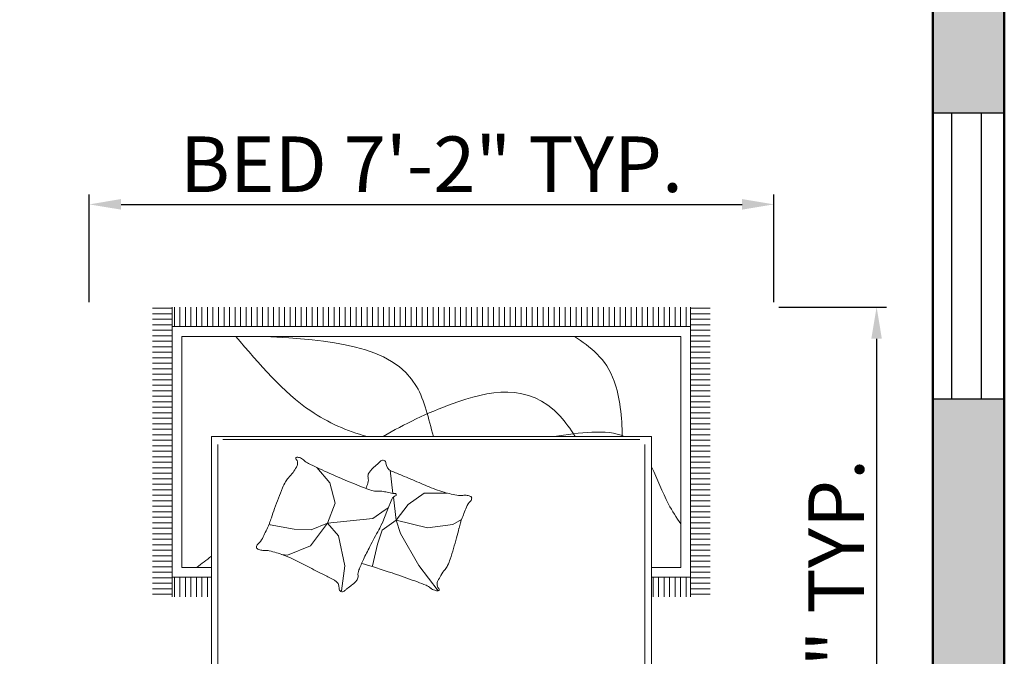
# Model space of a CAD drawing. Units: inches. Extents: x -7 to 1228, y -146 to 1091.
# Tile 84 of 88: x 1003 to 1127, y 611 to 691. Entities that reach past the tile are written whole.
import ezdxf

# ---------------------------------------------------------------- set-up
doc = ezdxf.new("R2010")
doc.units = ezdxf.units.IN
for name, color, linetype, lineweight in [('A-ANNO-DIMS', 2, 'Continuous', 18), ('A-FURN', 8, 'Continuous', 18), ('A-GLAZ', 175, 'Continuous', 25), ('A-WALL', 7, 'Continuous', 50), ('A-WALL-PATT', 251, 'Continuous', 13)]:
    doc.layers.add(name, color=color, linetype=linetype, lineweight=lineweight)
doc.styles.add('DIM_FONT', font='SIMPLEX.shx', dxfattribs={"width": 0.8})
doc.styles.get("Standard").update_dxf_attribs({"font": 'arial.ttf'})
doc.dimstyles.new('ISO-25', dxfattribs={"dimtxt": 7, "dimasz": 4, "dimexe": 1.25, "dimexo": 0.625, "dimtad": 1, "dimdec": 1, "dimlunit": 3, "dimtxsty": 'Standard', "dimcen": 2.5, "dimadec": 0, "dimazin": 0, "dimtfac": 1, "dimtdec": 1, "dimtmove": 1, "dimatfit": 3, "dimfxl": 1, "dimarcsym": 0})

# ---------------------------------------------------------------- blocks, each defined once
blk = doc.blocks.new('A$C4F634EDD')
for p, q in [((0.5, 0.5295), (0.5, 2.6295)), ((2.3, 2.6295), (2.3, 0.5295)), ((0.5258, 2.121), (0.5258, 0.5617)), ((2.2716, 0.5617), (2.2716, 1.7136)), ((0.2586, 1.1753), (0.3386, 1.1753)), ((0.3386, 0), (0.3386, 1.1852)), ((0.3486, 1.1052), (0.3486, 1.1852)), ((0.3711, 1.1052), (0.3711, 1.1852)), ((0.3936, 1.1052), (0.3936, 1.1852)), ((0.4161, 1.1052), (0.4161, 1.1852)), ((0.4386, 1.1052), (0.4386, 1.1852)), ((0.4611, 1.1052), (0.4611, 1.1852)), ((0.4836, 1.1052), (0.4836, 1.1852)), ((2.3061, 1.1052), (2.3061, 1.1852)), ((2.3286, 1.1052), (2.3286, 1.1852)), ((2.3511, 1.1052), (2.3511, 1.1852)), ((2.3736, 1.1052), (2.3736, 1.1852)), ((2.3961, 1.1052), (2.3961, 1.1852)), ((2.4186, 1.1052), (2.4186, 1.1852)), ((2.4411, 1.1052), (2.4411, 1.1852)), ((2.4588, 1.1852), (2.4588, 0)), ((2.4588, 1.1753), (2.5388, 1.1753)), ((0.2586, 1.1528), (0.3386, 1.1528)), ((0.2586, 1.1303), (0.3386, 1.1303)), ((1.031, 1.1612), (1.0448, 1.0581)), ((1.4276, 1.1611), (1.3484, 1.0571)), ((2.4588, 1.1528), (2.5388, 1.1528)), ((2.4588, 1.1303), (2.5388, 1.1303)), ((0.2586, 1.1078), (0.3386, 1.1078)), ((0.3386, 1.1052), (0.5, 1.1052)), ((2.3, 1.1052), (2.4588, 1.1052)), ((2.4588, 1.1078), (2.5388, 1.1078)), ((0.2586, 1.0853), (0.3386, 1.0853)), ((0.2586, 1.0628), (0.3386, 1.0628)), ((0.3786, 1.0652), (0.5, 1.0652)), ((0.3786, 0.12), (0.3786, 1.0652)), ((1.0448, 1.0581), (1.019, 0.936)), ((1.1784, 0.9702), (1.1586, 1.0591)), ((1.3484, 1.0571), (1.2733, 0.9268)), ((2.3, 1.0652), (2.4188, 1.0652)), ((2.4188, 1.0652), (2.4188, 0.12)), ((2.4588, 1.0853), (2.5388, 1.0853)), ((2.4588, 1.0628), (2.5388, 1.0628)), ((0.2586, 1.0403), (0.3386, 1.0403)), ((0.2586, 1.0178), (0.3386, 1.0178)), ((0.8108, 1.0151), (0.7868, 1.0117)), ((0.9054, 0.9773), (0.8108, 1.0151)), ((2.4588, 1.0403), (2.5388, 1.0403)), ((2.4588, 1.0178), (2.5388, 1.0178)), ((0.2586, 0.9953), (0.3386, 0.9953)), ((0.2586, 0.9728), (0.3386, 0.9728)), ((0.9743, 0.8845), (0.9054, 0.9773)), ((1.1982, 0.9129), (1.1784, 0.9702)), ((2.4588, 0.9953), (2.5388, 0.9953)), ((2.4588, 0.9728), (2.5388, 0.9728)), ((0.2586, 0.9503), (0.3386, 0.9503)), ((0.2586, 0.9278), (0.3386, 0.9278)), ((1.019, 0.936), (0.9743, 0.8845)), ((1.2733, 0.9268), (1.2555, 0.8715)), ((2.4588, 0.9503), (2.5388, 0.9503)), ((2.4588, 0.9278), (2.5388, 0.9278)), ((0.2586, 0.9053), (0.3386, 0.9053)), ((0.7403, 0.8913), (0.737, 0.8849)), ((0.8384, 0.9085), (0.7403, 0.8913)), ((0.9072, 0.912), (0.8384, 0.9085)), ((0.9743, 0.8845), (0.9072, 0.912)), ((1.2555, 0.8715), (1.1982, 0.9129)), ((1.2555, 0.8715), (1.384, 0.9031)), ((1.384, 0.9031), (1.4868, 0.8892)), ((1.4868, 0.8892), (1.5228, 0.8692)), ((2.4588, 0.9053), (2.5388, 0.9053)), ((0.2586, 0.8828), (0.3386, 0.8828)), ((0.2586, 0.8603), (0.3386, 0.8603)), ((0.9743, 0.8845), (1.0052, 0.802)), ((0.9743, 0.8845), (1.16, 0.8656)), ((1.16, 0.8656), (1.2099, 0.8295)), ((1.1973, 0.8853), (1.2203, 0.829)), ((1.2555, 0.8715), (1.2437, 0.7773)), ((1.2555, 0.8715), (1.3049, 0.8082)), ((2.4588, 0.8828), (2.5388, 0.8828)), ((2.4588, 0.8603), (2.5388, 0.8603)), ((0.2586, 0.8378), (0.3386, 0.8378)), ((0.2586, 0.8153), (0.3386, 0.8153)), ((1.2099, 0.8295), (1.222, 0.8209)), ((1.2203, 0.829), (1.2381, 0.7855)), ((1.3049, 0.8082), (1.3701, 0.7608)), ((2.4588, 0.8378), (2.5388, 0.8378)), ((2.4588, 0.8153), (2.5388, 0.8153)), ((0.2586, 0.7928), (0.3386, 0.7928)), ((0.2586, 0.7703), (0.3386, 0.7703)), ((1.0052, 0.802), (0.9846, 0.7194)), ((2.4588, 0.7928), (2.5388, 0.7928)), ((2.4588, 0.7703), (2.5388, 0.7703)), ((0.2586, 0.7478), (0.3386, 0.7478)), ((0.2586, 0.7253), (0.3386, 0.7253)), ((1.2419, 0.7626), (1.23, 0.668)), ((1.3701, 0.7608), (1.463, 0.7608)), ((2.4588, 0.7478), (2.5388, 0.7478)), ((2.4588, 0.7253), (2.5388, 0.7253)), ((0.2586, 0.7028), (0.3386, 0.7028)), ((0.9846, 0.7194), (0.931, 0.6569)), ((2.4588, 0.7028), (2.5388, 0.7028)), ((0.2586, 0.6803), (0.3386, 0.6803)), ((0.2586, 0.6578), (0.3386, 0.6578)), ((2.4588, 0.6803), (2.5388, 0.6803)), ((2.4588, 0.6578), (2.5388, 0.6578)), ((0.2586, 0.6353), (0.3386, 0.6353)), ((0.2586, 0.6128), (0.3386, 0.6128)), ((2.4588, 0.6353), (2.5388, 0.6353)), ((2.4588, 0.6128), (2.5388, 0.6128)), ((0.2586, 0.5903), (0.3386, 0.5903)), ((0.2586, 0.5678), (0.3386, 0.5678)), ((2.4588, 0.5903), (2.5388, 0.5903)), ((2.4588, 0.5678), (2.5388, 0.5678)), ((0.2586, 0.5453), (0.3386, 0.5453)), ((2.3, 0.5295), (0.5, 0.5295)), ((0.5458, 0.5417), (2.2516, 0.5417)), ((2.4588, 0.5453), (2.5388, 0.5453)), ((0.2586, 0.5228), (0.3386, 0.5228)), ((0.2586, 0.5003), (0.3386, 0.5003)), ((2.4588, 0.5228), (2.5388, 0.5228)), ((2.4588, 0.5003), (2.5388, 0.5003)), ((0.2586, 0.4778), (0.3386, 0.4778)), ((0.2586, 0.4553), (0.3386, 0.4553)), ((2.4588, 0.4778), (2.5388, 0.4778)), ((2.4588, 0.4553), (2.5388, 0.4553)), ((0.2586, 0.4328), (0.3386, 0.4328)), ((0.2586, 0.4103), (0.3386, 0.4103)), ((2.4588, 0.4328), (2.5388, 0.4328)), ((2.4588, 0.4103), (2.5388, 0.4103)), ((0.2586, 0.3878), (0.3386, 0.3878)), ((0.2586, 0.3653), (0.3386, 0.3653)), ((2.4588, 0.3878), (2.5388, 0.3878)), ((2.4588, 0.3653), (2.5388, 0.3653)), ((0.2586, 0.3428), (0.3386, 0.3428)), ((2.4588, 0.3428), (2.5388, 0.3428)), ((0.2586, 0.3203), (0.3386, 0.3203)), ((0.2586, 0.2978), (0.3386, 0.2978)), ((2.4588, 0.3203), (2.5388, 0.3203)), ((2.4588, 0.2978), (2.5388, 0.2978)), ((0.2586, 0.2753), (0.3386, 0.2753)), ((0.2586, 0.2528), (0.3386, 0.2528)), ((2.4588, 0.2753), (2.5388, 0.2753)), ((2.4588, 0.2528), (2.5388, 0.2528)), ((0.2586, 0.2303), (0.3386, 0.2303)), ((0.2586, 0.2078), (0.3386, 0.2078)), ((2.4588, 0.2303), (2.5388, 0.2303)), ((2.4588, 0.2078), (2.5388, 0.2078)), ((0.2586, 0.1853), (0.3386, 0.1853)), ((0.2586, 0.1628), (0.3386, 0.1628)), ((2.4588, 0.1853), (2.5388, 0.1853)), ((2.4588, 0.1628), (2.5388, 0.1628)), ((0.2586, 0.1403), (0.3386, 0.1403)), ((2.4588, 0.1403), (2.5388, 0.1403)), ((0.2586, 0.1178), (0.3386, 0.1178)), ((0.2586, 0.0953), (0.3386, 0.0953)), ((2.4188, 0.12), (0.3786, 0.12)), ((2.4588, 0.1178), (2.5388, 0.1178)), ((2.4588, 0.0953), (2.5388, 0.0953)), ((0.2586, 0.0728), (0.3386, 0.0728)), ((0.2586, 0.0503), (0.3386, 0.0503)), ((2.4588, 0.08), (0.3386, 0.08)), ((0.3486, 0), (0.3486, 0.08)), ((0.3711, 0), (0.3711, 0.08)), ((0.3936, 0), (0.3936, 0.08)), ((0.4161, 0), (0.4161, 0.08)), ((0.4386, 0), (0.4386, 0.08)), ((0.4611, 0), (0.4611, 0.08)), ((0.4836, 0), (0.4836, 0.08)), ((0.5061, 0), (0.5061, 0.08)), ((0.5286, 0), (0.5286, 0.08)), ((0.5511, 0), (0.5511, 0.08)), ((0.5736, 0), (0.5736, 0.08)), ((0.5961, 0), (0.5961, 0.08)), ((0.6186, 0), (0.6186, 0.08)), ((0.6411, 0), (0.6411, 0.08)), ((0.6636, 0), (0.6636, 0.08)), ((0.6861, 0), (0.6861, 0.08)), ((0.7086, 0), (0.7086, 0.08)), ((0.7311, 0), (0.7311, 0.08)), ((0.7536, 0), (0.7536, 0.08)), ((0.7761, 0), (0.7761, 0.08)), ((0.7986, 0), (0.7986, 0.08)), ((0.8211, 0), (0.8211, 0.08)), ((0.8436, 0), (0.8436, 0.08)), ((0.8661, 0), (0.8661, 0.08)), ((0.8886, 0), (0.8886, 0.08)), ((0.9111, 0), (0.9111, 0.08)), ((0.9336, 0), (0.9336, 0.08)), ((0.9561, 0), (0.9561, 0.08)), ((0.9786, 0), (0.9786, 0.08)), ((1.0011, 0), (1.0011, 0.08)), ((1.0236, 0), (1.0236, 0.08)), ((1.0461, 0), (1.0461, 0.08)), ((1.0686, 0), (1.0686, 0.08)), ((1.0911, 0), (1.0911, 0.08)), ((1.1136, 0), (1.1136, 0.08)), ((1.1361, 0), (1.1361, 0.08)), ((1.1586, 0), (1.1586, 0.08)), ((1.1811, 0), (1.1811, 0.08)), ((1.2036, 0), (1.2036, 0.08)), ((1.2261, 0), (1.2261, 0.08)), ((1.2486, 0), (1.2486, 0.08)), ((1.2711, 0), (1.2711, 0.08)), ((1.2936, 0), (1.2936, 0.08)), ((1.3161, 0), (1.3161, 0.08)), ((1.3386, 0), (1.3386, 0.08)), ((1.3611, 0), (1.3611, 0.08)), ((1.3836, 0), (1.3836, 0.08)), ((1.4061, 0), (1.4061, 0.08)), ((1.4286, 0), (1.4286, 0.08)), ((1.4511, 0), (1.4511, 0.08)), ((1.4736, 0), (1.4736, 0.08)), ((1.4961, 0), (1.4961, 0.08)), ((1.5186, 0), (1.5186, 0.08)), ((1.5411, 0), (1.5411, 0.08)), ((1.5636, 0), (1.5636, 0.08)), ((1.5861, 0), (1.5861, 0.08)), ((1.6086, 0), (1.6086, 0.08)), ((1.6311, 0), (1.6311, 0.08)), ((1.6536, 0), (1.6536, 0.08)), ((1.6761, 0), (1.6761, 0.08)), ((1.6986, 0), (1.6986, 0.08)), ((1.7211, 0), (1.7211, 0.08)), ((1.7436, 0), (1.7436, 0.08)), ((1.7661, 0), (1.7661, 0.08)), ((1.7886, 0), (1.7886, 0.08)), ((1.8111, 0), (1.8111, 0.08)), ((1.8336, 0), (1.8336, 0.08)), ((1.8561, 0), (1.8561, 0.08)), ((1.8786, 0), (1.8786, 0.08)), ((1.9011, 0), (1.9011, 0.08)), ((1.9236, 0), (1.9236, 0.08)), ((1.9461, 0), (1.9461, 0.08)), ((1.9686, 0), (1.9686, 0.08)), ((1.9911, 0), (1.9911, 0.08)), ((2.0136, 0), (2.0136, 0.08)), ((2.0361, 0), (2.0361, 0.08)), ((2.0586, 0), (2.0586, 0.08)), ((2.0811, 0), (2.0811, 0.08)), ((2.1036, 0), (2.1036, 0.08)), ((2.1261, 0), (2.1261, 0.08)), ((2.1486, 0), (2.1486, 0.08)), ((2.1711, 0), (2.1711, 0.08)), ((2.1936, 0), (2.1936, 0.08)), ((2.2161, 0), (2.2161, 0.08)), ((2.2386, 0), (2.2386, 0.08)), ((2.2611, 0), (2.2611, 0.08)), ((2.2836, 0), (2.2836, 0.08)), ((2.3061, 0), (2.3061, 0.08)), ((2.3286, 0), (2.3286, 0.08)), ((2.3511, 0), (2.3511, 0.08)), ((2.3736, 0), (2.3736, 0.08)), ((2.3961, 0), (2.3961, 0.08)), ((2.4186, 0), (2.4186, 0.08)), ((2.4411, 0), (2.4411, 0.08)), ((2.4588, 0.0728), (2.5388, 0.0728)), ((2.4588, 0.0503), (2.5388, 0.0503)), ((0.2586, 0.0278), (0.3386, 0.0278)), ((0.2586, 0.0053), (0.3386, 0.0053)), ((2.4588, 0.0278), (2.5388, 0.0278)), ((2.4588, 0.0053), (2.5388, 0.0053))]:
    blk.add_line(p, q)
for centre, radius, start, end in [((0.9863, 1.1494), 0.0359, 297.2902, 3.2455), ((1.0348, 1.1521), 0.0127, 51.1864, 183.2455), ((0.9991, 1.1077), 0.0697, 45.8726, 51.1864), ((1.0791, 1.1902), 0.0452, 225.8726, 232.4713), ((1.2846, 1.4577), 0.3825, 232.4713, 233.7837), ((0.6683, 0.6162), 0.6605, 52.7849, 53.7837), ((0.9362, 0.9689), 0.2176, 46.4776, 52.7849), ((1.0543, 1.9106), 0.8371, 290.1287, 292.7069), ((1.3469, 1.2115), 0.0792, 292.7069, 308.5854), ((1.4338, 1.1026), 0.0601, 110.3452, 128.5854), ((1.4251, 1.1259), 0.0352, 86.0516, 110.3452), ((1.4996, 1.1284), 0.0771, 169.5926, 177.2714), ((1.4378, 1.1314), 0.0153, 177.2714, 194.5709), ((1.4611, 1.1374), 0.0393, 194.5709, 206.8179), ((1.4376, 1.1398), 0.0142, 126.5792, 169.5926), ((1.4273, 1.1567), 0.00443, 13.2808, 86.0516), ((1.4254, 1.1562), 0.0063, 306.5792, 13.2808), ((1.8575, -0.7096), 2.0162, 116.4147, 117.4999), ((-0.4173, 3.8699), 3.0972, 296.4147, 297.2902), ((1.0327, 1.0706), 0.0774, 35.8936, 46.4776), ((1.0771, 1.1027), 0.0226, 351.9508, 35.8936), ((1.1449, 1.0931), 0.0458, 171.9508, 202.4162), ((0.2266, 4.0657), 3.145, 286.6085, 289.0836), ((-0.4107, 5.9078), 5.0942, 289.0836, 290.1287), ((1.7401, 1.2785), 0.352, 206.8179, 210.9056), ((1.6045, 1.1973), 0.194, 210.9056, 219.7005), ((-1.8336, 6.2238), 5.8383, 297.49208, 297.84822), ((3.744, -4.3336), 6.1019, 117.49986, 117.84822), ((2.032, 1.4591), 1.0054, 202.4162, 205.0529), ((1.0922, 1.1636), 0.1166, 280.7366, 286.6085), ((1.3929, 1.0217), 0.081, 26.0735, 39.7005), ((1.2892, 0.9709), 0.1965, 17.8396, 26.0735), ((0.6422, 1.4168), 0.43, 282.6252, 290.7486), ((0.5736, 1.5979), 0.6236, 290.7486, 297.4921), ((2.6493, 1.7476), 1.6868, 205.0529, 207.0884), ((-0.4304, 0.4175), 2.003, 15.2625, 17.8396), ((0.6894, 0.9832), 0.0058, 121.6917, 179.0386), ((0.7004, 0.983), 0.0168, 179.0386, 229.4914), ((0.7131, 0.9448), 0.0509, 103.0402, 121.6917), ((0.6405, 0.9128), 0.0755, 26.3332, 49.4914), ((0.7152, 0.9361), 0.0599, 86.6119, 103.0402), ((0.7224, 1.0587), 0.063, 266.6119, 282.6252), ((2.541, 1.6922), 1.5652, 207.0884, 209.936), ((-1.6775, -0.2344), 2.6619, 25.1732, 26.3332), ((-0.0881, 0.5109), 1.6481, 13.841, 15.2625), ((0.5689, 0.8213), 0.1798, 20.7081, 25.1732), ((0.9989, 0.8042), 0.2143, 22.2355, 29.936), ((2.0418, 1.0357), 0.5454, 193.841, 196.3122), ((0.2268, 0.692), 0.5454, 18.2369, 20.7081), ((2.3102, 1.3785), 1.6481, 198.2369, 199.6584), ((1.6908, 0.933), 0.1798, 196.3122, 200.7773), ((4.0115, 1.8135), 2.6619, 200.7773, 201.9373), ((2.6444, 1.4979), 2.003, 199.6584, 202.2355), ((1.6124, 0.8472), 0.0755, 201.9373, 225.0955), ((1.2594, 0.7942), 0.0231, 202.2355, 252.8133), ((1.2512, 0.7678), 0.00467, 289.3799, 72.8133), ((1.5721, 0.3449), 0.43, 98.2293, 106.3527), ((1.5195, 0.708), 0.063, 82.216, 98.2293), ((1.5362, 0.8298), 0.0599, 262.216, 278.6443), ((1.5375, 0.8209), 0.0509, 278.6443, 297.2959), ((1.5473, 0.7819), 0.0168, 354.6428, 45.0955), ((1.5582, 0.7808), 0.0058, 297.2959, 354.6428), ((0.9722, 0.8143), 0.1965, 202.2355, 210.4694), ((2.2689, -2.1899), 3.145, 111.0043, 113.4795), ((0.1831, 0.4093), 1.0054, 18.0203, 19.3448), ((1.1834, 0.6373), 0.1166, 98.1216, 111.0043), ((1.1763, 0.687), 0.0663, 85.4882, 98.1216), ((1.1871, 0.8241), 0.0712, 265.4882, 277.6784), ((1.1727, 0.9313), 0.1794, 277.6784, 284.8807), ((1.2689, 0.569), 0.1955, 97.9822, 104.8807), ((1.2465, 0.729), 0.034, 85.7407, 97.9822), ((1.2497, 0.772), 0.0092, 265.7407, 289.3799), ((3.6722, -4.6377), 5.8383, 113.0962, 113.45234), ((1.6266, 0.159), 0.6236, 106.3527, 113.0962), ((0.8727, 0.7557), 0.081, 210.4694, 224.0964), ((0.6752, 0.5644), 0.194, 35.3015, 44.0964), ((3.0455, -3.9778), 5.0942, 113.4795, 114.5246), ((1.0957, 0.7061), 0.0458, 347.5549, 18.0203), ((1.1625, 0.6914), 0.0226, 167.5549, 211.4977), ((2.4404, -2.1823), 3.0972, 112.0188, 112.8944), ((0.5234, 2.5582), 2.0162, 292.0188, 293.104), ((-1.0798, 6.3161), 6.1019, 293.10398, 293.45234), ((0.5462, 0.4731), 0.352, 31.2138, 35.3015), ((0.8136, 0.6351), 0.0393, 18.9668, 31.2138), ((0.8364, 0.6429), 0.0153, 1.6673, 18.9668), ((1.2784, -0.1047), 0.8371, 114.5246, 117.1028), ((1.2092, 0.72), 0.0774, 211.4977, 222.0817), ((1.3133, 0.814), 0.2176, 222.0817, 228.389), ((1.6074, 1.1451), 0.6605, 228.389, 229.3878), ((1.2495, 0.6379), 0.0359, 112.8944, 178.8496), ((0.8506, 0.6191), 0.0063, 130.9751, 197.6767), ((0.8488, 0.6185), 0.00443, 197.6767, 270.4475), ((0.8372, 0.6345), 0.0142, 310.9751, 353.9885), ((0.8486, 0.6493), 0.0352, 270.4475, 294.7411), ((0.7746, 0.6411), 0.0771, 353.9885, 1.6673), ((0.8382, 0.6719), 0.0601, 294.7411, 312.9813), ((0.9332, 0.57), 0.0792, 117.1028, 132.9813), ((0.9284, 0.3533), 0.3825, 48.0754, 49.3878), ((1.1538, 0.6043), 0.0452, 41.4767, 48.0754), ((1.2399, 0.6804), 0.0697, 221.4767, 226.7905), ((1.2009, 0.6389), 0.0127, 226.7905, 358.8496)]:
    blk.add_arc(centre, radius, start, end)
for points in [[(0.4393, 1.0652), (0.4595, 1.05), (0.4798, 1.0348), (0.5, 1.0195)], [(1.9003, 0.5295), (2.0065, 0.514), (2.1132, 0.4978), (2.1894, 0.5295)]]:
    blk.add_open_spline(points, degree=3)
for points, knots in [([(2.3, 0.6535), (2.3236, 0.7026), (2.3554, 0.7914), (2.4015, 0.8608), (2.4188, 0.8868)], [1893.525221, 1893.525221, 1893.525221, 1893.525221, 2051.902476, 2146.74457, 2146.74457, 2146.74457, 2146.74457]), ([(0.5992, 0.12), (0.6957, 0.2341), (0.8523, 0.4189), (1.0536, 0.5069), (1.136, 0.5295)], [0, 0, 0, 0, 432.822832, 701.445452, 701.445452, 701.445452, 701.445452]), ([(0.7187, 0.12), (0.9791, 0.1362), (1.326, 0.1577), (1.3868, 0.4574), (1.408, 0.5295)], [0, 0, 0, 0, 653.160442, 870.050857, 870.050857, 870.050857, 870.050857]), ([(1.2016, 0.5295), (1.2892, 0.479), (1.5144, 0.3684), (1.8265, 0.2994), (1.9681, 0.4992), (1.9875, 0.5295)], [936.534237, 936.534237, 936.534237, 936.534237, 1243.285375, 1683.261222, 1758.254386, 1758.254386, 1758.254386, 1758.254386]), ([(2.1796, 0.5295), (2.1798, 0.4519), (2.1548, 0.2369), (2.0487, 0.164), (1.9846, 0.12)], [2202.034493, 2202.034493, 2202.034493, 2202.034493, 2357.807635, 2594.446174, 2594.446174, 2594.446174, 2594.446174])]:
    blk.add_open_spline(points, degree=3, knots=knots)
at = {"style": 'DIM_FONT', "width": 0.8, "flags": 9}
for tag, p in [('YSIZE', (0.5, 2.6295)), ('XSIZE', (0.5, 2.6295)), ('XSIZE', (2.2985, 2.6295)), ('YSIZE', (2.2985, 2.6295))]:
    blk.add_attdef(tag, p, '', height=0.0005, dxfattribs=at)
blk = doc.blocks.new('WIN-36')
for p, q in [((0, 36), (0, 0)), ((9, 36), (0, 36)), ((2.34, 36), (2.34, 0)), ((6.14, 0), (6.14, 36)), ((9, 0), (9, 36)), ((0, 0), (9, 0)), ((2.34, 0), (6.14, 0))]:
    blk.add_line(p, q)
blk = doc.blocks.new('*D26')
at = {"layer": 'A-ANNO-DIMS', "color": 0, "lineweight": -2, "transparency": 16777216}
for p, q in [((1011.76, 655.6), (1011.76, 669.15)), ((1097.98, 655.6), (1097.98, 669.15)), ((1015.76, 667.9), (1093.98, 667.9))]:
    blk.add_line(p, q, dxfattribs=at)
at = {"layer": 'A-ANNO-DIMS', "color": 0, "transparency": 16777216}
for points in [[(1015.76, 668.57), (1015.76, 667.24), (1011.76, 667.9)], [(1093.98, 668.57), (1093.98, 667.24), (1097.98, 667.9)]]:
    blk.add_solid(points, dxfattribs=at)
at = {"layer": 'Defpoints', "color": 0, "transparency": 16777216}
for p in [(1097.98, 667.9), (1011.76, 654.97), (1097.98, 654.97)]:
    blk.add_point(p, dxfattribs=at)
at = {"layer": 'A-ANNO-DIMS', "color": 0, "transparency": 16777216, "insert": (1054.87, 672.05), "char_height": 7, "attachment_point": 5}
blk.add_mtext('BED 7\'-2" TYP.', dxfattribs=at)
blk = doc.blocks.new('*D27')
at = {"layer": 'A-ANNO-DIMS', "color": 0, "lineweight": -2, "transparency": 16777216}
for p, q in [((1098.61, 654.97), (1112.17, 654.97)), ((1110.92, 650.97), (1110.92, 577.98)), ((1098.61, 573.98), (1112.17, 573.98))]:
    blk.add_line(p, q, dxfattribs=at)
at = {"layer": 'A-ANNO-DIMS', "color": 0, "transparency": 16777216}
for points in [[(1110.25, 650.97), (1111.58, 650.97), (1110.92, 654.97)], [(1110.25, 577.98), (1111.58, 577.98), (1110.92, 573.98)]]:
    blk.add_solid(points, dxfattribs=at)
at = {"layer": 'Defpoints', "color": 0, "transparency": 16777216}
for p in [(1097.98, 654.97), (1097.98, 573.98), (1110.92, 573.98)]:
    blk.add_point(p, dxfattribs=at)
at = {"layer": 'A-ANNO-DIMS', "color": 0, "transparency": 16777216, "insert": (1106.72, 614.48), "char_height": 7, "attachment_point": 5, "rotation": 90}
blk.add_mtext('6\'-9" TYP.', dxfattribs=at)

msp = doc.modelspace()

# ---------------------------------------------------------------- hatches: boundary and pattern name
at = {"layer": 'A-WALL-PATT'}
h = msp.add_hatch(color=256, dxfattribs=at)
h.dxf.hatch_style = 1
h.paths.add_polyline_path([(69, 568), (60, 568), (60, 493), (63.29, 493), (69, 493)])
h.paths.add_polyline_path([(69, 662.41), (60, 662.41), (60, 586), (69, 586)], flags=17)
h.paths.add_polyline_path([(69, 723), (184, 723), (184, 734), (179, 734), (179, 728), (69, 728), (69, 741.62), (60, 741.62), (60, 698.41), (69, 698.41)], flags=17)
h.paths.add_polyline_path([(69, 782), (231, 782), (231, 728), (231, 723), (231, 586), (236, 586), (236, 787), (69, 787), (69, 800.13), (60, 800.13), (60, 765.62), (69, 765.62)])
h.paths.add_polyline_path([(184, 842), (189, 842), (189, 848), (173, 848), (173, 842), (179, 842), (179, 787), (184, 787)])
h.paths.add_polyline_path([(118.22, 69), (69, 69), (69, 60), (118.22, 60)])
h.paths.add_polyline_path([(227, 69), (154.22, 69), (154.22, 60), (227, 60)])
h.paths.add_polyline_path([(236, 60), (232.71, 60), (227, 60), (227, 36), (236, 36)])
h.paths.add_polyline_path([(389, 60), (380, 60), (380, 36), (389, 36)])
h.paths.add_polyline_path([(384, 181), (380, 181), (380, 115), (380, 78), (384, 78)])
h.paths.add_polyline_path([(380, 115), (334.55, 115), (334.55, 109), (380, 109)])
h.paths.add_polyline_path([(274.55, 115), (236, 115), (236, 201), (232.71, 201), (231, 201), (231, 78), (236, 78), (236, 109), (274.55, 109)])
h.paths.add_polyline_path([(69, 123), (60, 123), (60, 78), (69, 78)])
h.paths.add_polyline_path([(69, 201), (60, 201), (60, 159), (69, 159)])
h.paths.add_polyline_path([(143, 219), (69, 219), (69, 213), (143, 213)], flags=17)
h.paths.add_polyline_path([(189, 219), (184, 219), (184, 274), (231, 274), (231, 219), (236, 219), (236, 279), (184, 279), (184, 297), (179, 297), (179, 279), (69, 279), (69, 290.91), (60, 290.91), (60, 262.18), (69, 262.18), (69, 274), (179, 274), (179, 219), (173, 219), (173, 213), (189, 213)])
h.paths.add_polyline_path([(69, 238.18), (60, 238.18), (60, 219), (69, 219)], flags=17)
h.paths.add_polyline_path([(69, 333), (60, 333), (60, 314.91), (69, 314.91), (69, 316.96)])
h.paths.add_polyline_path([(190, 338), (184, 338), (69, 338), (69, 333), (179, 333), (179, 327), (184, 327), (184, 333.02), (190, 333.05)])
h.paths.add_polyline_path([(69, 386.81), (60, 386.81), (60, 351), (69, 351)])
h.paths.add_polyline_path([(69, 475), (60, 475), (60, 422.81), (69, 422.81)])
h.paths.add_polyline_path([(236, 475), (231, 475), (231, 351.24), (236, 351.24)])
h.paths.add_polyline_path([(384, 475), (380, 475), (380, 362), (384, 362)])
h.paths.add_polyline_path([(547, 307), (439, 307), (439, 356), (445, 356), (445, 362), (433, 362), (433, 307), (380, 307), (380, 244), (380, 241), (384, 241), (384, 301), (433, 301), (433, 277), (439, 277), (439, 301), (547, 301)])
h.paths.add_polyline_path([(547, 241), (439, 241), (439, 247), (433, 247), (433, 235), (547, 235)])
h.paths.add_polyline_path([(450, 69), (440.29, 69), (424.89, 69), (389, 69), (389, 60), (450, 60)])
h.paths.add_polyline_path([(547, 69), (486, 69), (486, 60), (547, 60)])
h.paths.add_polyline_path([(556, 148.27), (547, 148.27), (547, 78), (556, 78)])
h.paths.add_polyline_path([(556, 223), (547, 223), (547, 195), (547, 184.27), (556, 184.27)])
h.paths.add_polyline_path([(556, 311.19), (547, 311.19), (547, 273.08), (556, 273.08)])
h.paths.add_polyline_path([(556, 344), (552.71, 344), (547, 344), (547, 335.19), (556, 335.19)])
h.paths.add_polyline_path([(556, 249.08), (547, 249.08), (547, 241), (556, 241)])
h.paths.add_polyline_path([(547, 362), (475, 362), (475, 356), (547, 356)], flags=0)
h.paths.add_polyline_path([(556, 399.62), (547, 399.62), (547, 362), (556, 362)])
h.paths.add_polyline_path([(556, 475), (547, 475), (547, 435.62), (556, 435.62)])
h.paths.add_polyline_path([(547, 493), (389, 493), (389, 487), (547, 487)])
h.paths.add_polyline_path([(380, 493), (278, 493), (278, 487), (380, 487)])
h.paths.add_polyline_path([(227, 493), (69, 493), (69, 487), (227, 487)])
h.paths.add_polyline_path([(643, 122.44), (634, 122.44), (634, 78), (643, 78)])
h.paths.add_polyline_path([(702.5, 69), (692.79, 69), (677.39, 69), (643, 69), (643, 60), (702.5, 60)])
h.paths.add_polyline_path([(798, 69), (738.5, 69), (738.5, 60), (798, 60)])
h.paths.add_polyline_path([(807, 60), (803.71, 60), (798, 60), (798, 36), (807, 36)])
h.paths.add_polyline_path([(807, 109), (846.75, 109), (846.75, 115), (807, 115), (807, 159), (802, 159), (802, 78), (807, 78)])
h.paths.add_polyline_path([(807, 201), (802, 201), (802, 195), (807, 195)])
h.paths.add_polyline_path([(643, 201), (634, 201), (634, 158.44), (643, 158.44)])
h.paths.add_polyline_path([(756, 225), (751, 225), (751, 219), (643, 219), (643, 213), (756, 213)])
h.paths.add_polyline_path([(643, 240.85), (634, 240.85), (634, 219), (643, 219)])
h.paths.add_polyline_path([(643, 274), (643, 288.63), (634, 288.63), (634, 264.85), (643, 264.85)])
h.paths.add_polyline_path([(802, 279), (756, 279), (756, 297), (751, 297), (751, 279), (643, 279), (643, 274), (751, 274), (751, 255), (756, 255), (756, 274), (802, 274)])
h.paths.add_polyline_path([(807, 333), (803.71, 333), (802, 333), (802, 279), (802, 274), (802, 219), (807, 219)])
h.paths.add_polyline_path([(956, 182), (951, 182), (951, 115), (906.75, 115), (906.75, 109), (951, 109), (951, 78), (956, 78)])
h.paths.add_polyline_path([(960, 60), (951, 60), (951, 36), (960, 36)])
h.paths.add_polyline_path([(1021, 69), (1005.78, 69), (960, 69), (960, 60), (1021, 60)])
h.paths.add_polyline_path([(956, 224), (951, 224), (951, 218), (956, 218)])
h.paths.add_polyline_path([(956, 302), (1004, 302), (1004, 278), (1010, 278), (1010, 302), (1118, 302), (1118, 290.81), (1127, 290.81), (1127, 326.97), (1118, 326.97), (1118, 320.97), (1118, 307), (1010, 307), (1010, 356), (1016, 356), (1016, 362), (1004, 362), (1004, 307), (951, 307), (951, 244), (951, 242), (954.29, 242), (956, 242)])
h.paths.add_polyline_path([(643, 333), (634, 333), (634, 312.63), (643, 312.63), (643, 316.96)])
h.paths.add_polyline_path([(756, 338), (643, 338), (643, 333), (751, 333), (751, 327), (756, 327)])
h.paths.add_polyline_path([(643, 388), (634, 388), (634, 351), (643, 351)])
h.paths.add_polyline_path([(807, 357), (802, 357), (802, 351), (807, 351)])
h.paths.add_polyline_path([(807, 475), (802, 475), (802, 393), (807, 393)])
h.paths.add_polyline_path([(643, 475), (634, 475), (634, 424), (643, 424)])
h.paths.add_polyline_path([(798, 493), (643, 493), (643, 487), (798, 487)])
h.paths.add_polyline_path([(634, 493), (556, 493), (556, 487), (634, 487)])
h.paths.add_polyline_path([(813, 493), (807, 493), (807, 487), (813, 487)])
h.paths.add_polyline_path([(951, 493), (849, 493), (849, 487), (951, 487)])
h.paths.add_polyline_path([(956, 484), (951, 484), (951, 374), (956, 374)])
h.paths.add_polyline_path([(1109, 493), (969, 493), (969, 487), (1109, 487)])
h.paths.add_polyline_path([(1127, 484), (1118, 484), (1118, 450.64), (1127, 450.64)])
h.paths.add_polyline_path([(1127, 414.64), (1118, 414.64), (1118, 365), (1127, 365)])
h.paths.add_polyline_path([(1109, 362), (1046, 362), (1046, 356), (1109, 356)], flags=17)
h.paths.add_polyline_path([(1127, 356), (1123.45, 356), (1118, 356), (1118, 350.97), (1127, 350.97)], flags=0)
h.paths.add_polyline_path([(1127, 266.81), (1118, 266.81), (1118, 262.36), (1118, 242), (1127, 242)], flags=17)
h.paths.add_polyline_path([(1118, 242), (1010, 242), (1010, 248), (1004, 248), (1004, 237), (1118, 237)])
h.paths.add_polyline_path([(1127, 224), (1118, 224), (1118, 170), (1127, 170)])
h.paths.add_polyline_path([(1127, 134), (1118, 134), (1118, 78), (1127, 78)])
h.paths.add_polyline_path([(1118, 69), (1057, 69), (1057, 60), (1118, 60)])
h.paths.add_polyline_path([(227, 571.55), (227, 574), (69, 574), (69, 568), (227, 568)])
h.paths.add_polyline_path([(380, 571.55), (380, 574), (278, 574), (278, 568), (380, 568)])
h.paths.add_polyline_path([(242, 574), (236, 574), (236, 568), (242, 568)])
h.paths.add_polyline_path([(547, 571.55), (547, 574), (389, 574), (389, 568), (547, 568)])
h.paths.add_polyline_path([(384, 733), (380, 733), (380, 586), (384, 586)])
h.paths.add_polyline_path([(556, 646), (634, 646), (634, 655), (547, 655), (547, 586), (556, 586)])
h.paths.add_polyline_path([(634, 574), (556, 574), (556, 568), (634, 568)])
h.paths.add_polyline_path([(643, 655), (634, 655), (634, 586), (643, 586)])
h.paths.add_polyline_path([(798, 574), (643, 574), (643, 568), (798, 568)])
h.paths.add_polyline_path([(643, 663.85), (634, 663.85), (634, 655), (643, 655)])
h.paths.add_polyline_path([(556, 676.97), (547, 676.97), (547, 655), (556, 655)])
h.paths.add_polyline_path([(556, 733), (547, 733), (547, 712.97), (556, 712.97)])
h.paths.add_polyline_path([(643, 710), (634, 710), (634, 699.85), (643, 699.85)])
h.paths.add_polyline_path([(807, 668), (802, 668), (802, 586), (807, 586)])
h.paths.add_polyline_path([(951, 574), (849, 574), (849, 568), (951, 568)])
h.paths.add_polyline_path([(956, 691), (951, 691), (951, 577), (956, 577)])
h.paths.add_polyline_path([(1109, 574), (969, 574), (969, 568), (1109, 568)])
h.paths.add_polyline_path([(1127, 643.4), (1118, 643.4), (1118, 577), (1127, 577)])
h.paths.add_polyline_path([(1127, 568), (1123.45, 568), (1118, 568), (1118, 493), (1127, 493)])
h.paths.add_polyline_path([(1127, 733), (1118, 733), (1118, 679.4), (1127, 679.4)])
h.paths.add_polyline_path([(1127, 777.35), (1118, 777.35), (1118, 770.04), (1118, 751), (1127, 751)], flags=17)
h.paths.add_polyline_path([(1118, 751), (1010, 751), (1010, 757), (1004, 757), (1004, 745), (1118, 745)])
h.paths.add_polyline_path([(956, 811), (1004, 811), (1004, 787), (1010, 787), (1010, 811), (1017.87, 811), (1017.87, 811.63, -0.414214), (1018.25, 812), (1031.98, 812, -0.414214), (1032.35, 811.63), (1032.35, 811), (1118, 811), (1118, 801.35), (1127, 801.35), (1127, 834.69), (1118, 834.69), (1118, 830.24), (1118, 817), (1010, 817), (1010, 866), (1016, 866), (1016, 872), (1004, 872), (1004, 817), (956, 817), (956, 866), (951, 866), (951, 751), (954.29, 751), (956, 751)])
h.paths.add_polyline_path([(1118, 872), (1046, 872), (1046, 866), (1118, 866)], flags=17)
h.paths.add_polyline_path([(1127, 924.71), (1118, 924.71), (1118, 884), (1127, 884)])
h.paths.add_polyline_path([(1127, 866), (1123.71, 866), (1118, 866), (1118, 858.69), (1127, 858.69)], flags=17)
h.paths.add_polyline_path([(956, 983), (951, 983), (951, 952), (807, 952), (807, 983), (802, 983), (802, 902), (807, 902), (807, 946), (951, 946), (951, 884), (956, 884)])
h.paths.add_polyline_path([(807, 842), (802, 842), (802, 787), (756, 787), (756, 806), (751, 806), (751, 787), (643, 787), (643, 782), (751, 782), (751, 764), (756, 764), (756, 782), (802, 782), (802, 728), (807, 728)])
h.paths.add_polyline_path([(756, 848), (643, 848), (643, 842), (751, 842), (751, 836), (756, 836)])
h.paths.add_polyline_path([(756, 734), (751, 734), (751, 728), (643, 728), (643, 723), (756, 723)])
h.paths.add_polyline_path([(643, 749.79), (634, 749.79), (634, 728), (637.29, 728), (643, 728)])
h.paths.add_polyline_path([(643, 805.41), (634, 805.41), (634, 773.79), (643, 773.79)])
h.paths.add_polyline_path([(643, 896.66), (634, 896.66), (634, 860), (637.29, 860), (643, 860)])
h.paths.add_polyline_path([(643, 842), (634, 842), (634, 829.41), (643, 829.41)])
h.paths.add_polyline_path([(643, 983), (634, 983), (634, 932.66), (643, 932.66)])
h.paths.add_polyline_path([(1127, 983), (1118, 983), (1118, 960.71), (1127, 960.71)])
h.paths.add_polyline_path([(1118, 1001), (1077.53, 1001), (1077.53, 992), (1118, 992)])
h.paths.add_polyline_path([(1041.53, 1001), (960, 1001), (960, 992), (1041.53, 992)])
h.paths.add_polyline_path([(960, 1025), (951, 1025), (951, 1001), (954.29, 1001), (960, 1001)])
h.paths.add_polyline_path([(807, 1025), (798, 1025), (798, 1001), (807, 1001)])
h.paths.add_polyline_path([(798, 1001), (738.5, 1001), (738.5, 992), (798, 992)])
h.paths.add_polyline_path([(702.5, 1001), (643, 1001), (643, 992), (702.5, 992)])
h.paths.add_polyline_path([(547, 1001), (499.11, 1001), (499.11, 992), (547, 992)])
h.paths.add_polyline_path([(463.11, 1001), (389, 1001), (389, 992), (463.11, 992)])
h.paths.add_polyline_path([(389, 1025), (380, 1025), (380, 1022), (380, 1001), (383.29, 1001), (389, 1001)])
h.paths.add_polyline_path([(236, 1025), (227, 1025), (227, 1001), (236, 1001)])
h.paths.add_polyline_path([(236, 983), (231, 983), (231, 860), (236, 860)])
h.paths.add_polyline_path([(274.55, 952), (236, 952), (236, 946), (274.55, 946)])
h.paths.add_polyline_path([(380, 952), (334.55, 952), (334.55, 946), (380, 946)])
h.paths.add_polyline_path([(384, 983), (380, 983), (380, 884), (383.29, 884), (384, 884)])
h.paths.add_polyline_path([(227, 1001), (155.01, 1001), (155.01, 992), (162.87, 992), (227, 992)])
h.paths.add_polyline_path([(119.01, 1001), (69, 1001), (69, 992), (119.01, 992)])
h.paths.add_polyline_path([(69, 983), (60, 983), (60, 922.99), (69, 922.99)])
h.paths.add_polyline_path([(69, 886.99), (60, 886.99), (60, 860), (63.29, 860), (69, 860)])
h.paths.add_polyline_path([(143, 848), (69, 848), (69, 842), (143, 842)])

# ---------------------------------------------------------------- linework, layer by layer
at = {"layer": 'A-WALL'}
for p, q in [((1127, 60), (1127, 1001)), ((1118, 307), (1118, 811))]:
    msp.add_line(p, q, dxfattribs=at)

# ---------------------------------------------------------------- block references
at = {"layer": 'A-FURN', "xscale": -30.79356024027943, "yscale": 30.79356024027943, "zscale": 30.79356024027943, "rotation": 180}
msp.add_blockref('A$C4F634EDD', (1011.76, 654.97), dxfattribs=at)
at = {"layer": 'A-GLAZ'}
msp.add_blockref('WIN-36', (1118, 643.4), dxfattribs=at)

# ---------------------------------------------------------------- dimensions: what is measured, and where the dimension line sits
at = {"layer": 'A-ANNO-DIMS'}
dim = msp.add_linear_dim(base=(1097.98, 667.9), p1=(1011.76, 654.97), p2=(1097.98, 654.97), text='BED <> TYP.', dimstyle='ISO-25', override={"dimdec": 1, "dimlfac": 1, "dimrnd": 0, "dimzin": 1, "dimdsep": 46, "dimlunit": 4, "dimfrac": 2}, dxfattribs=at)
dim.commit()
dim.dimension.update_dxf_attribs({"geometry": '*D26', "text_midpoint": (1054.87, 672.05)})
dim = msp.add_linear_dim(base=(1110.92, 573.98), p1=(1097.98, 654.97), p2=(1097.98, 573.98), angle=270, text='<> TYP.', dimstyle='ISO-25', override={"dimdec": 1, "dimlfac": 1, "dimrnd": 0, "dimzin": 1, "dimdsep": 46, "dimlunit": 4, "dimfrac": 2}, dxfattribs=at)
dim.commit()
dim.dimension.update_dxf_attribs({"geometry": '*D27', "text_midpoint": (1106.72, 614.48)})

doc.saveas('drawing.dxf')
